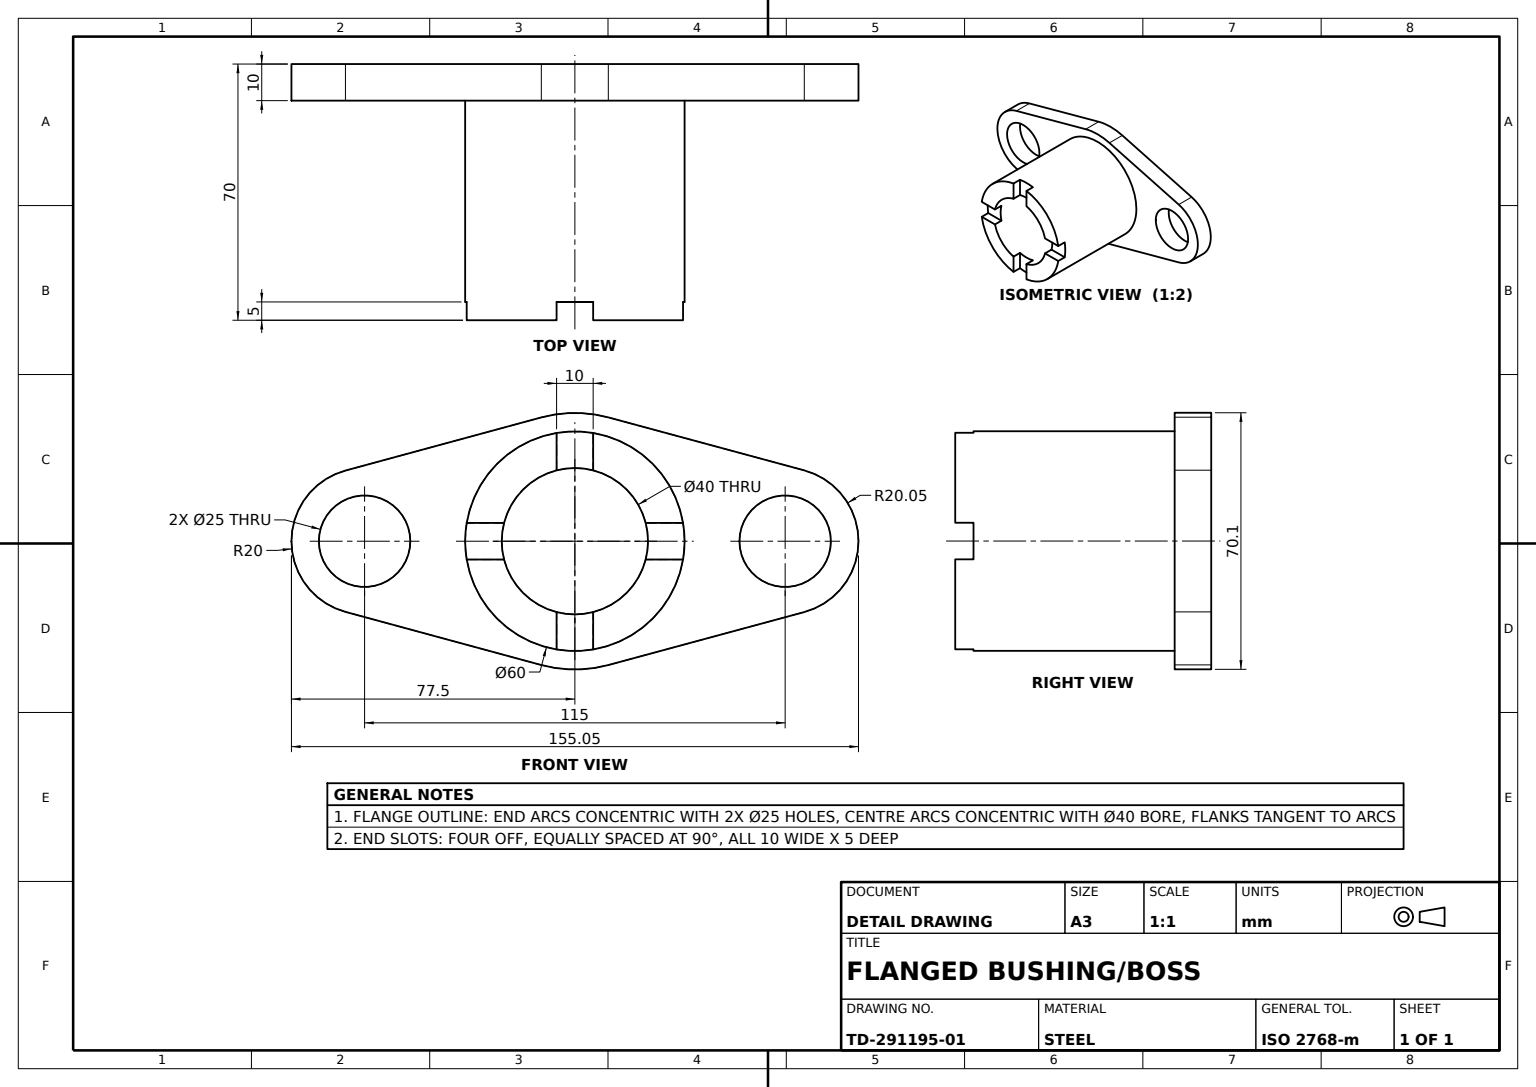
from build123d import *

# Parameters (mm, degrees)
FLANGE_PLATE_DEPTH      = 10
CYLINDER_BOSS_SKETCH_R  = 30
CYLINDER_BOSS_DEPTH     = 60
BORE_SKETCH_R           = 20
THROUGH_BORE_DEPTH      = 70
END_SLOTS_SKETCH_W      = 10
END_SLOTS_SKETCH_H      = 12.639410213
END_SLOTS_SKETCH_H_2    = 13.280913302
END_SLOTS_SKETCH_W_2    = 15.451741121
END_SLOTS_SKETCH_H_3    = 10
END_SLOTS_SKETCH_W_3    = 12.65016047
END_SLOTS_4X_DEPTH      = 5
MOUNTING_HOLES_SKETCH_R = 12.5
MOUNTING_HOLES_2X_DEPTH = 10


with BuildPart() as part:
    # Flange Plate Sketch → Flange Plate (new body)
    with BuildSketch(Plane.XY):
        with BuildLine():
            Line((9.143774129, 33.837267894), (62.730690194, 19.356587648))
            ThreePointArc((62.730690194, 19.356587648), (77.550875425, 0), (62.730690194, -19.356587648))
            Line((62.730690194, -19.356587648), (9.143774129, -33.837267894))
            ThreePointArc((9.143774129, -33.837267894), (-0.016117163, -35.050949261), (-9.174888429, -33.828844588))
            Line((-9.174888429, -33.828844588), (-62.735128416, -19.302506721))
            ThreePointArc((-62.735128416, -19.302506721), (-77.49983338, 0), (-62.735128416, 19.302506721))
            Line((-62.735128416, 19.302506721), (-9.174888429, 33.828844588))
            ThreePointArc((-9.174888429, 33.828844588), (-0.016117163, 35.050949261), (9.143774129, 33.837267894))
        make_face()
    extrude(amount=FLANGE_PLATE_DEPTH)

    # Cylinder Boss Sketch → Cylinder Boss (add)
    with BuildSketch(Plane.XY.offset(10)):
        Circle(CYLINDER_BOSS_SKETCH_R)
    extrude(amount=CYLINDER_BOSS_DEPTH)

    # Bore Sketch → Through Bore (cut)
    with BuildSketch(Plane.XY.offset(70)):
        Circle(BORE_SKETCH_R)
    extrude(amount=-THROUGH_BORE_DEPTH, mode=Mode.SUBTRACT)

    # End Slots Sketch → End Slots 4x (cut)
    with BuildSketch(Plane.XY.offset(70)):
        with Locations((0, 23.680294894)):
            Rectangle(END_SLOTS_SKETCH_W, END_SLOTS_SKETCH_H)
        with Locations((0, -23.359543349)):
            Rectangle(END_SLOTS_SKETCH_W, END_SLOTS_SKETCH_H_2)
        with Locations((-22.27412944, 0)):
            Rectangle(END_SLOTS_SKETCH_W_2, END_SLOTS_SKETCH_H_3)
        with Locations((23.674919765, 0)):
            Rectangle(END_SLOTS_SKETCH_W_3, END_SLOTS_SKETCH_H_3)
    extrude(amount=-END_SLOTS_4X_DEPTH, mode=Mode.SUBTRACT)

    # Mounting Holes Sketch → Mounting Holes 2x (cut)
    with BuildSketch(Plane.XY.offset(10)):
        with Locations((-57.5, 0)):
            Circle(MOUNTING_HOLES_SKETCH_R)
        with Locations((57.5, 0)):
            Circle(MOUNTING_HOLES_SKETCH_R)
    extrude(amount=-MOUNTING_HOLES_2X_DEPTH, mode=Mode.SUBTRACT)


solid = part.part
